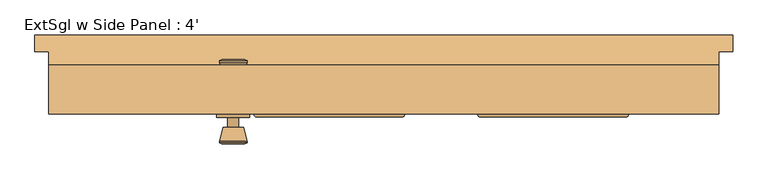
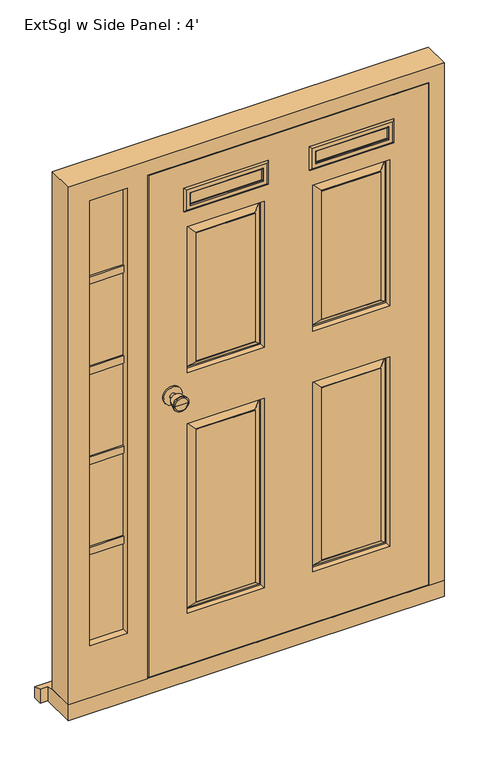
"""IFC4 building model written with IfcOpenShell, lengths in millimetres: door geometry, ExtSgl w Side Panel : 4'."""

from ifc_helpers import new_model, si_unit, point, frame, frame_2d, origin, place, context, project, spatial, polyline, circle_curve, ellipse_curve, trimmed, segment, composite_curve, outline, extrude, faceted_brep, source, transform, mapped, element, save
from ifc_brep_helpers import plane_surface, cylinder_surface, revolved_surface, advanced_brep


def extsgl_w_side_panel_4_38b62cc9(model_context):
    return source(origin(), model_context, "Body", "SolidModel", [
        advanced_brep(
        [(-493.3, -5.7, 1000.0), (-483.3, -5.7, 1000.0), (-503.3, -5.7, 1000.0), (-472.8241324, -54.7, 1000.0), (-493.3, -54.7, 1000.0), (-513.7758676, -54.7, 1000.0), (-468.3, -52.8721319, 1000.0), (-518.3, -52.8721319, 1000.0), (-468.3, -49.4084537, 1000.0), (-518.3, -49.4084537, 1000.0), (-474.663764, -24.7, 1000.0), (-511.936236, -24.7, 1000.0), (-483.3, -24.7, 1000.0), (-503.3, -24.7, 1000.0)],
        [
            (0, 1),
            (1, 2, circle_curve(frame((-493.3, -5.7, 1000.0), z_axis=(0.0, 1.0, 0.0), x_axis=(-1.0, 0.0, 0.0)), 10.0)),
            (2, 0),
            (2, 1, circle_curve(frame((-493.3, -5.7, 1000.0), z_axis=(0.0, 1.0, 0.0), x_axis=(-1.0, 0.0, 0.0)), 10.0)),
            (3, 4),
            (4, 5),
            (5, 3, circle_curve(frame((-493.3, -54.7, 1000.0), z_axis=(0.0, -1.0, 0.0), x_axis=(-1.0, 0.0, 0.0)), 20.4758676)),
            (3, 5, circle_curve(frame((-493.3, -54.7, 1000.0), z_axis=(0.0, -1.0, 0.0), x_axis=(-1.0, 0.0, 0.0)), 20.4758676)),
            (6, 3),
            (5, 7),
            (7, 6, circle_curve(frame((-493.3, -52.8721319, 1000.0), z_axis=(0.0, -1.0, 0.0), x_axis=(-1.0, 0.0, 0.0)), 25.0)),
            (6, 7, circle_curve(frame((-493.3, -52.8721319, 1000.0), z_axis=(0.0, -1.0, 0.0), x_axis=(-1.0, 0.0, 0.0)), 25.0)),
            (8, 6),
            (7, 9),
            (9, 8, circle_curve(frame((-493.3, -49.4084537, 1000.0), z_axis=(0.0, -1.0, 0.0), x_axis=(-1.0, 0.0, 0.0)), 25.0)),
            (8, 9, circle_curve(frame((-493.3, -49.4084537, 1000.0), z_axis=(0.0, -1.0, 0.0), x_axis=(-1.0, 0.0, 0.0)), 25.0)),
            (10, 8),
            (9, 11),
            (11, 10, circle_curve(frame((-493.3, -24.7, 1000.0), z_axis=(0.0, -1.0, 0.0), x_axis=(-1.0, 0.0, 0.0)), 18.636236)),
            (10, 11, circle_curve(frame((-493.3, -24.7, 1000.0), z_axis=(0.0, -1.0, 0.0), x_axis=(-1.0, 0.0, 0.0)), 18.636236)),
            (12, 10),
            (11, 13),
            (13, 12, circle_curve(frame((-493.3, -24.7, 1000.0), z_axis=(0.0, -1.0, 0.0), x_axis=(-1.0, 0.0, 0.0)), 10.0)),
            (12, 13, circle_curve(frame((-493.3, -24.7, 1000.0), z_axis=(0.0, -1.0, 0.0), x_axis=(-1.0, 0.0, 0.0)), 10.0)),
            (1, 12),
            (13, 2),
        ],
        [
            plane_surface(frame((-493.3, -5.7, 1000.0), z_axis=(0.0, 1.0, 0.0), x_axis=(-1.0, 0.0, 0.0))),
            plane_surface(frame((-493.3, -54.7, 1000.0), z_axis=(0.0, -1.0, 0.0), x_axis=(-1.0, 0.0, 0.0))),
            revolved_surface(polyline([(-513.7758676, -54.7, 1000.0), (-518.3, -52.8721319, 1000.0)]), (-493.3, -5.7, 1000.0), (0.0, 1.0, 0.0)),
            cylinder_surface(frame((-493.3, -5.7, 1000.0), z_axis=(0.0, 1.0, 0.0), x_axis=(-1.0, 0.0, 0.0)), 25.0),
            revolved_surface(polyline([(-518.3, -49.4084537, 1000.0), (-511.936236, -24.7, 1000.0)]), (-493.3, -5.7, 1000.0), (0.0, 1.0, 0.0)),
            plane_surface(frame((-493.3, -24.7, 1000.0), z_axis=(0.0, 1.0, 0.0), x_axis=(-1.0, 0.0, 0.0))),
            cylinder_surface(frame((-493.3, -5.7, 1000.0), z_axis=(0.0, 1.0, 0.0), x_axis=(-1.0, 0.0, 0.0)), 10.0),
        ],
        [
            (0, [[1, 2, 3]]),
            (0, [[-3, 4, -1]]),
            (1, [[5, 6, 7]]),
            (1, [[-6, -5, 8]]),
            (2, [[9, -7, 10, 11]]),
            (2, [[-10, -8, -9, 12]]),
            (3, [[13, -11, 14, 15]]),
            (3, [[-14, -12, -13, 16]]),
            (4, [[17, -15, 18, 19]]),
            (4, [[-18, -16, -17, 20]]),
            (5, [[21, -19, 22, 23]]),
            (5, [[-22, -20, -21, 24]]),
            (6, [[25, -23, 26, -2]]),
            (6, [[-26, -24, -25, -4]]),
        ],
    ),
        extrude(outline(composite_curve([segment(trimmed(circle_curve(frame_2d((1000.0, -493.3)), 30.0), [point((1000.0, -523.3))], [point((1000.0, -463.3))], False, "CARTESIAN"), True, "CONTINUOUS"), segment(trimmed(circle_curve(frame_2d((1000.0, -493.3)), 30.0), [point((1000.0, -463.3))], [point((1000.0, -523.3))], False, "CARTESIAN"), True, "CONTINUOUS")], self_intersect=False)), frame((0.0, -5.7, 0.0), z_axis=(0.0, 1.0, 0.0), x_axis=(0.0, 0.0, 1.0)), (0.0, 0.0, 1.0), 6.0),
        advanced_brep(
        [(-493.3, 50.3, 1000.0), (-503.3, 50.3, 1000.0), (-483.3, 50.3, 1000.0), (-472.8241324, 99.3, 1000.0), (-513.7758676, 99.3, 1000.0), (-493.3, 99.3, 1000.0), (-468.3, 97.4721319, 1000.0), (-518.3, 97.4721319, 1000.0), (-468.3, 94.0084537, 1000.0), (-518.3, 94.0084537, 1000.0), (-474.663764, 69.3, 1000.0), (-511.936236, 69.3, 1000.0), (-483.3, 69.3, 1000.0), (-503.3, 69.3, 1000.0)],
        [
            (0, 1),
            (1, 2, circle_curve(frame((-493.3, 50.3, 1000.0), z_axis=(0.0, -1.0, 0.0), x_axis=(-1.0, 0.0, 0.0)), 10.0)),
            (2, 0),
            (2, 1, circle_curve(frame((-493.3, 50.3, 1000.0), z_axis=(0.0, -1.0, 0.0), x_axis=(-1.0, 0.0, 0.0)), 10.0)),
            (3, 4, circle_curve(frame((-493.3, 99.3, 1000.0), z_axis=(0.0, 1.0, 0.0), x_axis=(-1.0, 0.0, 0.0)), 20.4758676)),
            (4, 5),
            (5, 3),
            (4, 3, circle_curve(frame((-493.3, 99.3, 1000.0), z_axis=(0.0, 1.0, 0.0), x_axis=(-1.0, 0.0, 0.0)), 20.4758676)),
            (6, 7, circle_curve(frame((-493.3, 97.4721319, 1000.0), z_axis=(0.0, 1.0, 0.0), x_axis=(-1.0, 0.0, 0.0)), 25.0)),
            (7, 4),
            (3, 6),
            (7, 6, circle_curve(frame((-493.3, 97.4721319, 1000.0), z_axis=(0.0, 1.0, 0.0), x_axis=(-1.0, 0.0, 0.0)), 25.0)),
            (8, 9, circle_curve(frame((-493.3, 94.0084537, 1000.0), z_axis=(0.0, 1.0, 0.0), x_axis=(-1.0, 0.0, 0.0)), 25.0)),
            (9, 7),
            (6, 8),
            (9, 8, circle_curve(frame((-493.3, 94.0084537, 1000.0), z_axis=(0.0, 1.0, 0.0), x_axis=(-1.0, 0.0, 0.0)), 25.0)),
            (10, 11, circle_curve(frame((-493.3, 69.3, 1000.0), z_axis=(0.0, 1.0, 0.0), x_axis=(-1.0, 0.0, 0.0)), 18.636236)),
            (11, 9),
            (8, 10),
            (11, 10, circle_curve(frame((-493.3, 69.3, 1000.0), z_axis=(0.0, 1.0, 0.0), x_axis=(-1.0, 0.0, 0.0)), 18.636236)),
            (12, 13, circle_curve(frame((-493.3, 69.3, 1000.0), z_axis=(0.0, 1.0, 0.0), x_axis=(-1.0, 0.0, 0.0)), 10.0)),
            (13, 11),
            (10, 12),
            (13, 12, circle_curve(frame((-493.3, 69.3, 1000.0), z_axis=(0.0, 1.0, 0.0), x_axis=(-1.0, 0.0, 0.0)), 10.0)),
            (1, 13),
            (12, 2),
        ],
        [
            plane_surface(frame((-493.3, 50.3, 1000.0), z_axis=(0.0, -1.0, 0.0), x_axis=(-1.0, 0.0, 0.0))),
            plane_surface(frame((-493.3, 99.3, 1000.0), z_axis=(0.0, 1.0, 0.0), x_axis=(-1.0, 0.0, 0.0))),
            revolved_surface(polyline([(-513.7758676, 99.3, 1000.0), (-518.3, 97.4721319, 1000.0)]), (-493.3, 50.3, 1000.0), (0.0, -1.0, 0.0)),
            cylinder_surface(frame((-493.3, 50.3, 1000.0), z_axis=(0.0, -1.0, 0.0), x_axis=(-1.0, 0.0, 0.0)), 25.0),
            revolved_surface(polyline([(-518.3, 94.0084537, 1000.0), (-511.936236, 69.3, 1000.0)]), (-493.3, 50.3, 1000.0), (0.0, -1.0, 0.0)),
            plane_surface(frame((-493.3, 69.3, 1000.0), z_axis=(0.0, -1.0, 0.0), x_axis=(-1.0, 0.0, 0.0))),
            cylinder_surface(frame((-493.3, 50.3, 1000.0), z_axis=(0.0, -1.0, 0.0), x_axis=(-1.0, 0.0, 0.0)), 10.0),
        ],
        [
            (0, [[1, 2, 3]]),
            (0, [[-3, 4, -1]]),
            (1, [[5, 6, 7]]),
            (1, [[8, -7, -6]]),
            (2, [[9, 10, -5, 11]]),
            (2, [[12, -11, -8, -10]]),
            (3, [[13, 14, -9, 15]]),
            (3, [[16, -15, -12, -14]]),
            (4, [[17, 18, -13, 19]]),
            (4, [[20, -19, -16, -18]]),
            (5, [[21, 22, -17, 23]]),
            (5, [[24, -23, -20, -22]]),
            (6, [[-2, 25, -21, 26]]),
            (6, [[-4, -26, -24, -25]]),
        ],
    ),
        extrude(outline(composite_curve([segment(trimmed(circle_curve(frame_2d((1000.0, -493.3)), 30.0), [point((1000.0, -523.3))], [point((1000.0, -463.3))], False, "CARTESIAN"), True, "CONTINUOUS"), segment(trimmed(circle_curve(frame_2d((1000.0, -493.3)), 30.0), [point((1000.0, -463.3))], [point((1000.0, -523.3))], False, "CARTESIAN"), True, "CONTINUOUS")], self_intersect=False)), frame((0.0, 44.3, 0.0), z_axis=(0.0, 1.0, 0.0), x_axis=(0.0, 0.0, 1.0)), (0.0, 0.0, 1.0), 6.0),
        faceted_brep([(319.7, 89.3, 54.5), (390.2, 89.3, 54.5), (390.2, 0.3, 54.5), (341.7, 0.3, 54.5), (341.7, 47.3, 54.5), (319.7, 47.3, 54.5), (319.7, 89.3, 1758.3), (-551.3, 89.3, 1758.3), (-551.3, 89.3, 54.5), (-829.0, 89.3, 54.5), (-829.0, 89.3, 1828.8), (390.2, 89.3, 1828.8), (-637.3, 89.3, 1758.3), (-758.5, 89.3, 1758.3), (-758.5, 89.3, 233.5), (-637.3, 89.3, 233.5), (390.2, 0.3, 1828.8), (-829.0, 0.3, 1828.8), (-829.0, 0.3, 54.5), (-573.3, 0.3, 54.5), (-573.3, 0.3, 1780.3), (341.7, 0.3, 1780.3), (-637.3, 0.3, 233.5), (-758.5, 0.3, 233.5), (-758.5, 0.3, 1758.3), (-637.3, 0.3, 1758.3), (341.7, 47.3, 1780.3), (-573.3, 47.3, 1780.3), (-573.3, 47.3, 54.5), (-551.3, 47.3, 54.5), (-551.3, 47.3, 1758.3), (319.7, 47.3, 1758.3), (-615.3, 47.3, 1780.3), (-780.5, 47.3, 1780.3), (-780.5, 47.3, 218.5), (-615.3, 47.3, 218.5), (-758.5, 47.3, 1758.3), (-637.3, 47.3, 1758.3), (-637.3, 47.3, 233.5), (-758.5, 47.3, 233.5), (-637.3, 23.3, 233.5), (-758.5, 23.3, 233.5), (-758.5, 23.3, 1758.3), (-637.3, 23.3, 1758.3), (-780.5, 23.3, 1780.3), (-780.5, 23.3, 218.5), (-615.3, 23.3, 218.5), (-615.3, 23.3, 1780.3)], [[[0, 1, 2, 3, 4, 5]], [[1, 0, 6, 7, 8, 9, 10, 11], [12, 13, 14, 15]], [[2, 1, 11, 16]], [[3, 2, 16, 17, 18, 19, 20, 21], [22, 23, 24, 25]], [[4, 3, 21, 26]], [[5, 4, 26, 27, 28, 29, 30, 31]], [[32, 33, 34, 35], [36, 37, 38, 39]], [[0, 5, 31, 6]], [[29, 8, 7, 30]], [[18, 9, 8, 29, 28, 19]], [[10, 9, 18, 17]], [[13, 36, 39, 14]], [[39, 38, 15, 14]], [[37, 12, 15, 38]], [[23, 22, 40, 41]], [[24, 23, 41, 42]], [[22, 25, 43, 40]], [[19, 28, 27, 20]], [[44, 45, 34, 33]], [[45, 46, 35, 34]], [[46, 47, 32, 35]], [[46, 45, 44, 47], [41, 40, 43, 42]], [[11, 10, 17, 16]], [[26, 21, 20, 27]], [[33, 32, 47, 44]], [[6, 31, 30, 7]], [[36, 13, 12, 37]], [[25, 24, 42, 43]]]),
        faceted_brep([(338.7, 0.3, 58.5), (338.7, 0.3, 1777.3), (-568.3, 0.3, 1777.3), (-568.3, 0.3, 58.5), (-36.3, 0.3, 1683.5), (213.7, 0.3, 1683.5), (213.7, 0.3, 1627.3), (-36.3, 0.3, 1627.3), (-443.3, 0.3, 1683.5), (-193.3, 0.3, 1683.5), (-193.3, 0.3, 1627.3), (-443.3, 0.3, 1627.3), (-193.3, 0.3, 883.5), (-193.3, 0.3, 233.5), (-443.3, 0.3, 233.5), (-443.3, 0.3, 883.5), (213.7, 0.3, 883.5), (213.7, 0.3, 233.5), (-36.3, 0.3, 233.5), (-36.3, 0.3, 883.5), (-193.3, 0.3, 1558.5), (-193.3, 0.3, 1058.5), (-443.3, 0.3, 1058.5), (-443.3, 0.3, 1558.5), (213.7, 0.3, 1558.5), (213.7, 0.3, 1058.5), (-36.3, 0.3, 1058.5), (-36.3, 0.3, 1558.5), (-223.3, 0.3, 263.5), (-223.3, 0.3, 853.5), (-413.3, 0.3, 853.5), (-413.3, 0.3, 263.5), (183.7, 0.3, 263.5), (183.7, 0.3, 853.5), (-6.3, 0.3, 853.5), (-6.3, 0.3, 263.5), (-223.3, 0.3, 1088.5), (-223.3, 0.3, 1528.5), (-413.3, 0.3, 1528.5), (-413.3, 0.3, 1088.5), (183.7, 0.3, 1088.5), (183.7, 0.3, 1528.5), (-6.3, 0.3, 1528.5), (-6.3, 0.3, 1088.5), (338.7, 44.3, 58.5), (-568.3, 44.3, 58.5), (-568.3, 44.3, 1777.3), (338.7, 44.3, 1777.3), (-36.3, 44.3, 1683.5), (-36.3, 44.3, 1627.3), (213.7, 44.3, 1627.3), (213.7, 44.3, 1683.5), (-443.3, 44.3, 1683.5), (-443.3, 44.3, 1627.3), (-193.3, 44.3, 1627.3), (-193.3, 44.3, 1683.5), (-36.3, 44.3, 883.5), (-36.3, 44.3, 233.5), (213.7, 44.3, 233.5), (213.7, 44.3, 883.5), (-443.3, 44.3, 883.5), (-443.3, 44.3, 233.5), (-193.3, 44.3, 233.5), (-193.3, 44.3, 883.5), (-36.3, 44.3, 1558.5), (-36.3, 44.3, 1058.5), (213.7, 44.3, 1058.5), (213.7, 44.3, 1558.5), (-443.3, 44.3, 1558.5), (-443.3, 44.3, 1058.5), (-193.3, 44.3, 1058.5), (-193.3, 44.3, 1558.5), (-6.3, 44.3, 263.5), (-6.3, 44.3, 853.5), (183.7, 44.3, 853.5), (183.7, 44.3, 263.5), (-413.3, 44.3, 263.5), (-413.3, 44.3, 853.5), (-223.3, 44.3, 853.5), (-223.3, 44.3, 263.5), (-6.3, 44.3, 1088.5), (-6.3, 44.3, 1528.5), (183.7, 44.3, 1528.5), (183.7, 44.3, 1088.5), (-413.3, 44.3, 1088.5), (-413.3, 44.3, 1528.5), (-223.3, 44.3, 1528.5), (-223.3, 44.3, 1088.5), (-33.3, 29.3, 880.5), (-33.3, 29.3, 236.5), (-8.3, 43.3, 855.5), (-8.3, 43.3, 261.5), (-28.3, 29.3, 241.5), (-28.3, 29.3, 875.5), (-6.3, 43.3, 263.5), (-6.3, 43.3, 853.5), (210.7, 29.3, 236.5), (185.7, 43.3, 261.5), (205.7, 29.3, 241.5), (183.7, 43.3, 263.5), (210.7, 29.3, 880.5), (185.7, 43.3, 855.5), (205.7, 29.3, 875.5), (183.7, 43.3, 853.5), (-440.3, 29.3, 880.5), (-440.3, 29.3, 236.5), (-415.3, 43.3, 855.5), (-415.3, 43.3, 261.5), (-435.3, 29.3, 241.5), (-435.3, 29.3, 875.5), (-413.3, 43.3, 263.5), (-413.3, 43.3, 853.5), (-196.3, 29.3, 236.5), (-221.3, 43.3, 261.5), (-201.3, 29.3, 241.5), (-223.3, 43.3, 263.5), (-196.3, 29.3, 880.5), (-221.3, 43.3, 855.5), (-201.3, 29.3, 875.5), (-223.3, 43.3, 853.5), (-223.3, 1.3, 263.5), (-223.3, 1.3, 853.5), (-201.3, 15.3, 241.5), (-201.3, 15.3, 875.5), (-221.3, 1.3, 855.5), (-221.3, 1.3, 261.5), (-196.3, 15.3, 880.5), (-196.3, 15.3, 236.5), (-413.3, 1.3, 853.5), (-435.3, 15.3, 875.5), (-415.3, 1.3, 855.5), (-440.3, 15.3, 880.5), (-413.3, 1.3, 263.5), (-435.3, 15.3, 241.5), (-415.3, 1.3, 261.5), (-440.3, 15.3, 236.5), (210.7, 15.3, 880.5), (210.7, 15.3, 236.5), (185.7, 1.3, 855.5), (185.7, 1.3, 261.5), (205.7, 15.3, 241.5), (205.7, 15.3, 875.5), (183.7, 1.3, 263.5), (183.7, 1.3, 853.5), (-33.3, 15.3, 236.5), (-8.3, 1.3, 261.5), (-28.3, 15.3, 241.5), (-6.3, 1.3, 263.5), (-33.3, 15.3, 880.5), (-8.3, 1.3, 855.5), (-28.3, 15.3, 875.5), (-6.3, 1.3, 853.5), (-6.3, 43.3, 1088.5), (-6.3, 43.3, 1528.5), (-28.3, 29.3, 1066.5), (-28.3, 29.3, 1550.5), (-8.3, 43.3, 1530.5), (-8.3, 43.3, 1086.5), (-33.3, 29.3, 1555.5), (-33.3, 29.3, 1061.5), (183.7, 43.3, 1528.5), (205.7, 29.3, 1550.5), (185.7, 43.3, 1530.5), (210.7, 29.3, 1555.5), (183.7, 43.3, 1088.5), (205.7, 29.3, 1066.5), (185.7, 43.3, 1086.5), (210.7, 29.3, 1061.5), (-413.3, 43.3, 1088.5), (-413.3, 43.3, 1528.5), (-435.3, 29.3, 1066.5), (-435.3, 29.3, 1550.5), (-415.3, 43.3, 1530.5), (-415.3, 43.3, 1086.5), (-440.3, 29.3, 1555.5), (-440.3, 29.3, 1061.5), (-223.3, 43.3, 1528.5), (-201.3, 29.3, 1550.5), (-221.3, 43.3, 1530.5), (-196.3, 29.3, 1555.5), (-223.3, 43.3, 1088.5), (-201.3, 29.3, 1066.5), (-221.3, 43.3, 1086.5), (-196.3, 29.3, 1061.5), (-223.3, 1.3, 1088.5), (-223.3, 1.3, 1528.5), (-201.3, 15.3, 1066.5), (-201.3, 15.3, 1550.5), (-221.3, 1.3, 1530.5), (-221.3, 1.3, 1086.5), (-196.3, 15.3, 1555.5), (-196.3, 15.3, 1061.5), (-413.3, 1.3, 1528.5), (-435.3, 15.3, 1550.5), (-415.3, 1.3, 1530.5), (-440.3, 15.3, 1555.5), (-413.3, 1.3, 1088.5), (-435.3, 15.3, 1066.5), (-415.3, 1.3, 1086.5), (-440.3, 15.3, 1061.5), (210.7, 15.3, 1555.5), (210.7, 15.3, 1061.5), (185.7, 1.3, 1530.5), (185.7, 1.3, 1086.5), (205.7, 15.3, 1066.5), (205.7, 15.3, 1550.5), (183.7, 1.3, 1088.5), (183.7, 1.3, 1528.5), (-33.3, 15.3, 1061.5), (-8.3, 1.3, 1086.5), (-28.3, 15.3, 1066.5), (-6.3, 1.3, 1088.5), (-33.3, 15.3, 1555.5), (-8.3, 1.3, 1530.5), (-28.3, 15.3, 1550.5), (-6.3, 1.3, 1528.5)], [[[0, 1, 2, 3], [4, 5, 6, 7], [8, 9, 10, 11], [12, 13, 14, 15], [16, 17, 18, 19], [20, 21, 22, 23], [24, 25, 26, 27]], [[28, 29, 30, 31]], [[32, 33, 34, 35]], [[36, 37, 38, 39]], [[40, 41, 42, 43]], [[44, 45, 46, 47], [48, 49, 50, 51], [52, 53, 54, 55], [56, 57, 58, 59], [60, 61, 62, 63], [64, 65, 66, 67], [68, 69, 70, 71]], [[72, 73, 74, 75]], [[76, 77, 78, 79]], [[80, 81, 82, 83]], [[84, 85, 86, 87]], [[1, 0, 44, 47]], [[2, 1, 47, 46]], [[3, 2, 46, 45]], [[0, 3, 45, 44]], [[4, 7, 49, 48]], [[7, 6, 50, 49]], [[6, 5, 51, 50]], [[5, 4, 48, 51]], [[8, 11, 53, 52]], [[11, 10, 54, 53]], [[10, 9, 55, 54]], [[9, 8, 52, 55]], [[88, 89, 57, 56]], [[90, 91, 92, 93]], [[72, 94, 95, 73]], [[57, 89, 96, 58]], [[92, 91, 97, 98]], [[94, 72, 75, 99]], [[58, 96, 100, 59]], [[98, 97, 101, 102]], [[99, 75, 74, 103]], [[88, 56, 59, 100]], [[89, 88, 100, 96], [93, 92, 98, 102]], [[90, 93, 102, 101]], [[91, 90, 101, 97], [95, 94, 99, 103]], [[73, 95, 103, 74]], [[104, 105, 61, 60]], [[106, 107, 108, 109]], [[76, 110, 111, 77]], [[61, 105, 112, 62]], [[108, 107, 113, 114]], [[110, 76, 79, 115]], [[62, 112, 116, 63]], [[114, 113, 117, 118]], [[115, 79, 78, 119]], [[104, 60, 63, 116]], [[105, 104, 116, 112], [109, 108, 114, 118]], [[106, 109, 118, 117]], [[107, 106, 117, 113], [111, 110, 115, 119]], [[77, 111, 119, 78]], [[120, 121, 29, 28]], [[122, 123, 124, 125]], [[12, 126, 127, 13]], [[29, 121, 128, 30]], [[124, 123, 129, 130]], [[126, 12, 15, 131]], [[30, 128, 132, 31]], [[130, 129, 133, 134]], [[131, 15, 14, 135]], [[120, 28, 31, 132]], [[125, 124, 130, 134], [121, 120, 132, 128]], [[122, 125, 134, 133]], [[127, 126, 131, 135], [123, 122, 133, 129]], [[13, 127, 135, 14]], [[136, 137, 17, 16]], [[138, 139, 140, 141]], [[32, 142, 143, 33]], [[17, 137, 144, 18]], [[140, 139, 145, 146]], [[142, 32, 35, 147]], [[18, 144, 148, 19]], [[146, 145, 149, 150]], [[147, 35, 34, 151]], [[136, 16, 19, 148]], [[137, 136, 148, 144], [141, 140, 146, 150]], [[138, 141, 150, 149]], [[139, 138, 149, 145], [143, 142, 147, 151]], [[33, 143, 151, 34]], [[152, 153, 81, 80]], [[154, 155, 156, 157]], [[64, 158, 159, 65]], [[81, 153, 160, 82]], [[156, 155, 161, 162]], [[158, 64, 67, 163]], [[82, 160, 164, 83]], [[162, 161, 165, 166]], [[163, 67, 66, 167]], [[152, 80, 83, 164]], [[157, 156, 162, 166], [153, 152, 164, 160]], [[154, 157, 166, 165]], [[159, 158, 163, 167], [155, 154, 165, 161]], [[65, 159, 167, 66]], [[168, 169, 85, 84]], [[170, 171, 172, 173]], [[68, 174, 175, 69]], [[85, 169, 176, 86]], [[172, 171, 177, 178]], [[174, 68, 71, 179]], [[86, 176, 180, 87]], [[178, 177, 181, 182]], [[179, 71, 70, 183]], [[168, 84, 87, 180]], [[173, 172, 178, 182], [169, 168, 180, 176]], [[170, 173, 182, 181]], [[175, 174, 179, 183], [171, 170, 181, 177]], [[69, 175, 183, 70]], [[184, 185, 37, 36]], [[186, 187, 188, 189]], [[20, 190, 191, 21]], [[37, 185, 192, 38]], [[188, 187, 193, 194]], [[190, 20, 23, 195]], [[38, 192, 196, 39]], [[194, 193, 197, 198]], [[195, 23, 22, 199]], [[184, 36, 39, 196]], [[189, 188, 194, 198], [185, 184, 196, 192]], [[186, 189, 198, 197]], [[191, 190, 195, 199], [187, 186, 197, 193]], [[21, 191, 199, 22]], [[200, 201, 25, 24]], [[202, 203, 204, 205]], [[40, 206, 207, 41]], [[25, 201, 208, 26]], [[204, 203, 209, 210]], [[206, 40, 43, 211]], [[26, 208, 212, 27]], [[210, 209, 213, 214]], [[211, 43, 42, 215]], [[200, 24, 27, 212]], [[201, 200, 212, 208], [205, 204, 210, 214]], [[202, 205, 214, 213]], [[203, 202, 213, 209], [207, 206, 211, 215]], [[41, 207, 215, 42]]]),
        faceted_brep([(415.2, 144.3, 0.0), (415.2, 144.3, 38.5947221), (415.2, 114.3, 47.2703282), (415.2, 114.3, 0.0), (-854.0, 144.3, 38.5947221), (-854.0, 144.3, 0.0), (-854.0, 114.3, 0.0), (-854.0, 114.3, 47.2703282), (390.2, 114.3, 0.0), (390.2, 0.3, 0.0), (-829.0, 0.3, 0.0), (-829.0, 114.3, 0.0), (-829.0, 114.3, 47.2703282), (-829.0, 89.3, 54.5), (390.2, 89.3, 54.5), (390.2, 114.3, 47.2703282), (-829.0, 0.3, 54.5), (390.2, 0.3, 54.5)], [[[0, 1, 2, 3]], [[4, 5, 6, 7]], [[5, 0, 3, 8, 9, 10, 11, 6]], [[1, 0, 5, 4]], [[1, 4, 7, 12, 13, 14, 15, 2]], [[13, 16, 17, 14]], [[16, 10, 9, 17]], [[12, 11, 10, 16, 13]], [[11, 12, 7, 6]], [[8, 15, 14, 17, 9]], [[15, 8, 3, 2]]]),
        extrude(outline(polyline([(213.7, 10.3), (-36.3, 10.3), (-36.3, 34.3), (213.7, 34.3), (213.7, 10.3)])), frame((0.0, 0.0, 1627.3), z_axis=(0.0, 0.0, 1.0), x_axis=(1.0, 0.0, 0.0)), (0.0, 0.0, 1.0), 56.2),
        extrude(outline(polyline([(-193.3, 10.3), (-443.3, 10.3), (-443.3, 34.3), (-193.3, 34.3), (-193.3, 10.3)])), frame((0.0, 0.0, 1627.3), z_axis=(0.0, 0.0, 1.0), x_axis=(1.0, 0.0, 0.0)), (0.0, 0.0, 1.0), 56.2),
        advanced_brep(
        [(-28.3, 48.3, 1675.5), (-28.3, 44.3, 1675.5), (-28.3, 44.3, 1635.3), (-28.3, 48.3, 1635.3), (-30.3, 50.3, 1677.5), (-30.3, 50.3, 1633.3), (-48.3, 45.3, 1695.5), (-43.3, 50.3, 1690.5), (-43.3, 50.3, 1620.3), (-48.3, 45.3, 1615.3), (-48.3, 34.3, 1695.5), (-48.3, 34.3, 1615.3), (-36.3, 44.3, 1683.5), (-36.3, 34.3, 1683.5), (-36.3, 34.3, 1627.3), (-36.3, 44.3, 1627.3), (205.7, 44.3, 1635.3), (205.7, 48.3, 1635.3), (207.7, 50.3, 1633.3), (220.7, 50.3, 1620.3), (225.7, 45.3, 1615.3), (225.7, 34.3, 1615.3), (213.7, 34.3, 1627.3), (213.7, 44.3, 1627.3), (205.7, 44.3, 1675.5), (205.7, 48.3, 1675.5), (207.7, 50.3, 1677.5), (220.7, 50.3, 1690.5), (225.7, 45.3, 1695.5), (225.7, 34.3, 1695.5), (213.7, 34.3, 1683.5), (213.7, 44.3, 1683.5)],
        [
            (0, 1),
            (1, 2),
            (2, 3),
            (3, 0),
            (4, 0, ellipse_curve(frame((-30.3, 48.3, 1677.5), z_axis=(-0.7071067811865475, 0.0, -0.7071067811865475), x_axis=(-0.7071067811865474, 0.0, 0.7071067811865476)), 2.8284271, 2.0)),
            (3, 5, ellipse_curve(frame((-30.3, 48.3, 1633.3), z_axis=(-0.7071067811865475, 0.0, 0.7071067811865475), x_axis=(0.7071067811865474, 0.0, 0.7071067811865476)), 2.8284271, 2.0)),
            (5, 4),
            (6, 7, ellipse_curve(frame((-43.3, 45.3, 1690.5), z_axis=(-0.7071067811865475, 0.0, -0.7071067811865475), x_axis=(-0.7071067811865474, 0.0, 0.7071067811865476)), 7.0710678, 5.0)),
            (7, 8),
            (8, 9, ellipse_curve(frame((-43.3, 45.3, 1620.3), z_axis=(-0.7071067811865475, 0.0, 0.7071067811865475), x_axis=(0.7071067811865474, 0.0, 0.7071067811865476)), 7.0710678, 5.0)),
            (9, 6),
            (10, 6),
            (9, 11),
            (11, 10),
            (12, 13),
            (13, 14),
            (14, 15),
            (15, 12),
            (2, 16),
            (16, 17),
            (17, 3),
            (17, 18, ellipse_curve(frame((207.7, 48.3, 1633.3), z_axis=(-0.7071067811865475, 0.0, -0.7071067811865475), x_axis=(-0.7071067811865476, 0.0, 0.7071067811865474)), 2.8284271, 2.0)),
            (18, 5),
            (8, 19),
            (19, 20, ellipse_curve(frame((220.7, 45.3, 1620.3), z_axis=(-0.7071067811865475, 0.0, -0.7071067811865475), x_axis=(-0.7071067811865476, 0.0, 0.7071067811865474)), 7.0710678, 5.0)),
            (20, 9),
            (20, 21),
            (21, 11),
            (14, 22),
            (22, 23),
            (23, 15),
            (16, 24),
            (24, 25),
            (25, 17),
            (25, 26, ellipse_curve(frame((207.7, 48.3, 1677.5), z_axis=(0.7071067811865475, 0.0, -0.7071067811865475), x_axis=(-0.7071067811865474, 0.0, -0.7071067811865476)), 2.8284271, 2.0)),
            (26, 18),
            (19, 27),
            (27, 28, ellipse_curve(frame((220.7, 45.3, 1690.5), z_axis=(0.7071067811865475, 0.0, -0.7071067811865475), x_axis=(-0.7071067811865474, 0.0, -0.7071067811865476)), 7.0710678, 5.0)),
            (28, 20),
            (28, 29),
            (29, 21),
            (22, 30),
            (30, 31),
            (31, 23),
            (24, 1),
            (0, 25),
            (4, 26),
            (7, 27),
            (6, 28),
            (10, 29),
            (13, 30),
            (12, 31),
        ],
        [
            plane_surface(frame((-28.3, 44.3, 1675.5), z_axis=(1.0, 0.0, 0.0), x_axis=(0.0, 0.0, -1.0))),
            cylinder_surface(frame((-30.3, 48.3, 1683.5), z_axis=(0.0, 0.0, 1.0), x_axis=(1.0, 0.0, 0.0)), 2.0),
            cylinder_surface(frame((-43.3, 45.3, 1683.5), z_axis=(0.0, 0.0, 1.0), x_axis=(1.0, 0.0, 0.0)), 5.0),
            plane_surface(frame((-48.3, 45.3, 1695.5), z_axis=(-1.0, 0.0, 0.0), x_axis=(0.0, 0.0, -1.0))),
            plane_surface(frame((-36.3, 34.3, 1683.5), z_axis=(1.0, 0.0, 0.0), x_axis=(0.0, 0.0, -1.0))),
            plane_surface(frame((-28.3, 44.3, 1635.3), z_axis=(0.0, 0.0, 1.0), x_axis=(1.0, 0.0, 0.0))),
            cylinder_surface(frame((-36.3, 48.3, 1633.3), z_axis=(-1.0, 0.0, 0.0), x_axis=(0.0, 0.0, 1.0)), 2.0),
            cylinder_surface(frame((-36.3, 45.3, 1620.3), z_axis=(-1.0, 0.0, 0.0), x_axis=(0.0, 0.0, 1.0)), 5.0),
            plane_surface(frame((-48.3, 45.3, 1615.3), z_axis=(0.0, 0.0, -1.0), x_axis=(1.0, 0.0, 0.0))),
            plane_surface(frame((-36.3, 34.3, 1627.3), z_axis=(0.0, 0.0, 1.0), x_axis=(1.0, 0.0, 0.0))),
            plane_surface(frame((205.7, 44.3, 1635.3), z_axis=(-1.0, 0.0, 0.0), x_axis=(0.0, 0.0, 1.0))),
            cylinder_surface(frame((207.7, 48.3, 1627.3), z_axis=(0.0, 0.0, -1.0), x_axis=(-1.0, 0.0, 0.0)), 2.0),
            cylinder_surface(frame((220.7, 45.3, 1627.3), z_axis=(0.0, 0.0, -1.0), x_axis=(-1.0, 0.0, 0.0)), 5.0),
            plane_surface(frame((225.7, 45.3, 1615.3), z_axis=(1.0, 0.0, 0.0), x_axis=(0.0, 0.0, 1.0))),
            plane_surface(frame((213.7, 34.3, 1627.3), z_axis=(-1.0, 0.0, 0.0), x_axis=(0.0, 0.0, 1.0))),
            plane_surface(frame((205.7, 44.3, 1675.5), z_axis=(0.0, 0.0, -1.0), x_axis=(-1.0, 0.0, 0.0))),
            cylinder_surface(frame((213.7, 48.3, 1677.5), z_axis=(1.0, 0.0, 0.0), x_axis=(0.0, 0.0, -1.0)), 2.0),
            plane_surface(frame((207.7, 50.3, 1677.5), z_axis=(0.0, 1.0, 0.0), x_axis=(-1.0, 0.0, 0.0))),
            cylinder_surface(frame((213.7, 45.3, 1690.5), z_axis=(1.0, 0.0, 0.0), x_axis=(0.0, 0.0, -1.0)), 5.0),
            plane_surface(frame((225.7, 45.3, 1695.5), z_axis=(0.0, 0.0, 1.0), x_axis=(-1.0, 0.0, 0.0))),
            plane_surface(frame((225.7, 34.3, 1695.5), z_axis=(0.0, -1.0, 0.0), x_axis=(-1.0, 0.0, 0.0))),
            plane_surface(frame((213.7, 34.3, 1683.5), z_axis=(0.0, 0.0, -1.0), x_axis=(-1.0, 0.0, 0.0))),
            plane_surface(frame((213.7, 44.3, 1683.5), z_axis=(0.0, -1.0, 0.0), x_axis=(-1.0, 0.0, 0.0))),
        ],
        [
            (0, [[1, 2, 3, 4]]),
            (1, [[5, -4, 6, 7]]),
            (2, [[8, 9, 10, 11]]),
            (3, [[12, -11, 13, 14]]),
            (4, [[15, 16, 17, 18]]),
            (5, [[-3, 19, 20, 21]]),
            (6, [[-6, -21, 22, 23]]),
            (7, [[-10, 24, 25, 26]]),
            (8, [[-13, -26, 27, 28]]),
            (9, [[-17, 29, 30, 31]]),
            (10, [[-20, 32, 33, 34]]),
            (11, [[-22, -34, 35, 36]]),
            (12, [[-25, 37, 38, 39]]),
            (13, [[-27, -39, 40, 41]]),
            (14, [[-30, 42, 43, 44]]),
            (15, [[-33, 45, -1, 46]]),
            (16, [[-35, -46, -5, 47]]),
            (17, [[48, -37, -24, -9], [-23, -36, -47, -7]]),
            (18, [[-38, -48, -8, 49]]),
            (19, [[-40, -49, -12, 50]]),
            (20, [[-28, -41, -50, -14], [51, -42, -29, -16]]),
            (21, [[-43, -51, -15, 52]]),
            (22, [[-31, -44, -52, -18], [-45, -32, -19, -2]]),
        ],
    ),
        advanced_brep(
        [(-435.3, 48.3, 1675.5), (-435.3, 44.3, 1675.5), (-435.3, 44.3, 1635.3), (-435.3, 48.3, 1635.3), (-437.3, 50.3, 1677.5), (-437.3, 50.3, 1633.3), (-455.3, 45.3, 1695.5), (-450.3, 50.3, 1690.5), (-450.3, 50.3, 1620.3), (-455.3, 45.3, 1615.3), (-455.3, 34.3, 1695.5), (-455.3, 34.3, 1615.3), (-443.3, 44.3, 1683.5), (-443.3, 34.3, 1683.5), (-443.3, 34.3, 1627.3), (-443.3, 44.3, 1627.3), (-201.3, 44.3, 1635.3), (-201.3, 48.3, 1635.3), (-199.3, 50.3, 1633.3), (-186.3, 50.3, 1620.3), (-181.3, 45.3, 1615.3), (-181.3, 34.3, 1615.3), (-193.3, 34.3, 1627.3), (-193.3, 44.3, 1627.3), (-201.3, 44.3, 1675.5), (-201.3, 48.3, 1675.5), (-199.3, 50.3, 1677.5), (-186.3, 50.3, 1690.5), (-181.3, 45.3, 1695.5), (-181.3, 34.3, 1695.5), (-193.3, 34.3, 1683.5), (-193.3, 44.3, 1683.5)],
        [
            (0, 1),
            (1, 2),
            (2, 3),
            (3, 0),
            (4, 0, ellipse_curve(frame((-437.3, 48.3, 1677.5), z_axis=(-0.7071067811865475, 0.0, -0.7071067811865475), x_axis=(-0.7071067811865474, 0.0, 0.7071067811865476)), 2.8284271, 2.0)),
            (3, 5, ellipse_curve(frame((-437.3, 48.3, 1633.3), z_axis=(-0.7071067811865475, 0.0, 0.7071067811865475), x_axis=(0.7071067811865474, 0.0, 0.7071067811865476)), 2.8284271, 2.0)),
            (5, 4),
            (6, 7, ellipse_curve(frame((-450.3, 45.3, 1690.5), z_axis=(-0.7071067811865475, 0.0, -0.7071067811865475), x_axis=(-0.7071067811865474, 0.0, 0.7071067811865476)), 7.0710678, 5.0)),
            (7, 8),
            (8, 9, ellipse_curve(frame((-450.3, 45.3, 1620.3), z_axis=(-0.7071067811865475, 0.0, 0.7071067811865475), x_axis=(0.7071067811865474, 0.0, 0.7071067811865476)), 7.0710678, 5.0)),
            (9, 6),
            (10, 6),
            (9, 11),
            (11, 10),
            (12, 13),
            (13, 14),
            (14, 15),
            (15, 12),
            (2, 16),
            (16, 17),
            (17, 3),
            (17, 18, ellipse_curve(frame((-199.3, 48.3, 1633.3), z_axis=(-0.7071067811865475, 0.0, -0.7071067811865475), x_axis=(-0.7071067811865476, 0.0, 0.7071067811865474)), 2.8284271, 2.0)),
            (18, 5),
            (8, 19),
            (19, 20, ellipse_curve(frame((-186.3, 45.3, 1620.3), z_axis=(-0.7071067811865475, 0.0, -0.7071067811865475), x_axis=(-0.7071067811865476, 0.0, 0.7071067811865474)), 7.0710678, 5.0)),
            (20, 9),
            (20, 21),
            (21, 11),
            (14, 22),
            (22, 23),
            (23, 15),
            (16, 24),
            (24, 25),
            (25, 17),
            (25, 26, ellipse_curve(frame((-199.3, 48.3, 1677.5), z_axis=(0.7071067811865475, 0.0, -0.7071067811865475), x_axis=(-0.7071067811865474, 0.0, -0.7071067811865476)), 2.8284271, 2.0)),
            (26, 18),
            (19, 27),
            (27, 28, ellipse_curve(frame((-186.3, 45.3, 1690.5), z_axis=(0.7071067811865475, 0.0, -0.7071067811865475), x_axis=(-0.7071067811865474, 0.0, -0.7071067811865476)), 7.0710678, 5.0)),
            (28, 20),
            (28, 29),
            (29, 21),
            (22, 30),
            (30, 31),
            (31, 23),
            (24, 1),
            (0, 25),
            (4, 26),
            (7, 27),
            (6, 28),
            (10, 29),
            (13, 30),
            (12, 31),
        ],
        [
            plane_surface(frame((-435.3, 44.3, 1675.5), z_axis=(1.0, 0.0, 0.0), x_axis=(0.0, 0.0, -1.0))),
            cylinder_surface(frame((-437.3, 48.3, 1683.5), z_axis=(0.0, 0.0, 1.0), x_axis=(1.0, 0.0, 0.0)), 2.0),
            cylinder_surface(frame((-450.3, 45.3, 1683.5), z_axis=(0.0, 0.0, 1.0), x_axis=(1.0, 0.0, 0.0)), 5.0),
            plane_surface(frame((-455.3, 45.3, 1695.5), z_axis=(-1.0, 0.0, 0.0), x_axis=(0.0, 0.0, -1.0))),
            plane_surface(frame((-443.3, 34.3, 1683.5), z_axis=(1.0, 0.0, 0.0), x_axis=(0.0, 0.0, -1.0))),
            plane_surface(frame((-435.3, 44.3, 1635.3), z_axis=(0.0, 0.0, 1.0), x_axis=(1.0, 0.0, 0.0))),
            cylinder_surface(frame((-443.3, 48.3, 1633.3), z_axis=(-1.0, 0.0, 0.0), x_axis=(0.0, 0.0, 1.0)), 2.0),
            cylinder_surface(frame((-443.3, 45.3, 1620.3), z_axis=(-1.0, 0.0, 0.0), x_axis=(0.0, 0.0, 1.0)), 5.0),
            plane_surface(frame((-455.3, 45.3, 1615.3), z_axis=(0.0, 0.0, -1.0), x_axis=(1.0, 0.0, 0.0))),
            plane_surface(frame((-443.3, 34.3, 1627.3), z_axis=(0.0, 0.0, 1.0), x_axis=(1.0, 0.0, 0.0))),
            plane_surface(frame((-201.3, 44.3, 1635.3), z_axis=(-1.0, 0.0, 0.0), x_axis=(0.0, 0.0, 1.0))),
            cylinder_surface(frame((-199.3, 48.3, 1627.3), z_axis=(0.0, 0.0, -1.0), x_axis=(-1.0, 0.0, 0.0)), 2.0),
            cylinder_surface(frame((-186.3, 45.3, 1627.3), z_axis=(0.0, 0.0, -1.0), x_axis=(-1.0, 0.0, 0.0)), 5.0),
            plane_surface(frame((-181.3, 45.3, 1615.3), z_axis=(1.0, 0.0, 0.0), x_axis=(0.0, 0.0, 1.0))),
            plane_surface(frame((-193.3, 34.3, 1627.3), z_axis=(-1.0, 0.0, 0.0), x_axis=(0.0, 0.0, 1.0))),
            plane_surface(frame((-201.3, 44.3, 1675.5), z_axis=(0.0, 0.0, -1.0), x_axis=(-1.0, 0.0, 0.0))),
            cylinder_surface(frame((-193.3, 48.3, 1677.5), z_axis=(1.0, 0.0, 0.0), x_axis=(0.0, 0.0, -1.0)), 2.0),
            plane_surface(frame((-199.3, 50.3, 1677.5), z_axis=(0.0, 1.0, 0.0), x_axis=(-1.0, 0.0, 0.0))),
            cylinder_surface(frame((-193.3, 45.3, 1690.5), z_axis=(1.0, 0.0, 0.0), x_axis=(0.0, 0.0, -1.0)), 5.0),
            plane_surface(frame((-181.3, 45.3, 1695.5), z_axis=(0.0, 0.0, 1.0), x_axis=(-1.0, 0.0, 0.0))),
            plane_surface(frame((-181.3, 34.3, 1695.5), z_axis=(0.0, -1.0, 0.0), x_axis=(-1.0, 0.0, 0.0))),
            plane_surface(frame((-193.3, 34.3, 1683.5), z_axis=(0.0, 0.0, -1.0), x_axis=(-1.0, 0.0, 0.0))),
            plane_surface(frame((-193.3, 44.3, 1683.5), z_axis=(0.0, -1.0, 0.0), x_axis=(-1.0, 0.0, 0.0))),
        ],
        [
            (0, [[1, 2, 3, 4]]),
            (1, [[5, -4, 6, 7]]),
            (2, [[8, 9, 10, 11]]),
            (3, [[12, -11, 13, 14]]),
            (4, [[15, 16, 17, 18]]),
            (5, [[-3, 19, 20, 21]]),
            (6, [[-6, -21, 22, 23]]),
            (7, [[-10, 24, 25, 26]]),
            (8, [[-13, -26, 27, 28]]),
            (9, [[-17, 29, 30, 31]]),
            (10, [[-20, 32, 33, 34]]),
            (11, [[-22, -34, 35, 36]]),
            (12, [[-25, 37, 38, 39]]),
            (13, [[-27, -39, 40, 41]]),
            (14, [[-30, 42, 43, 44]]),
            (15, [[-33, 45, -1, 46]]),
            (16, [[-35, -46, -5, 47]]),
            (17, [[48, -37, -24, -9], [-23, -36, -47, -7]]),
            (18, [[-38, -48, -8, 49]]),
            (19, [[-40, -49, -12, 50]]),
            (20, [[-28, -41, -50, -14], [51, -42, -29, -16]]),
            (21, [[-43, -51, -15, 52]]),
            (22, [[-31, -44, -52, -18], [-45, -32, -19, -2]]),
        ],
    ),
        advanced_brep(
        [(-201.3, -3.7, 1675.5), (-201.3, 0.3, 1675.5), (-201.3, 0.3, 1635.3), (-201.3, -3.7, 1635.3), (-199.3, -5.7, 1677.5), (-199.3, -5.7, 1633.3), (-181.3, -0.7, 1695.5), (-186.3, -5.7, 1690.5), (-186.3, -5.7, 1620.3), (-181.3, -0.7, 1615.3), (-181.3, 10.3, 1695.5), (-181.3, 10.3, 1615.3), (-193.3, 0.3, 1683.5), (-193.3, 10.3, 1683.5), (-193.3, 10.3, 1627.3), (-193.3, 0.3, 1627.3), (-435.3, 0.3, 1635.3), (-435.3, -3.7, 1635.3), (-437.3, -5.7, 1633.3), (-450.3, -5.7, 1620.3), (-455.3, -0.7, 1615.3), (-455.3, 10.3, 1615.3), (-443.3, 10.3, 1627.3), (-443.3, 0.3, 1627.3), (-435.3, 0.3, 1675.5), (-435.3, -3.7, 1675.5), (-437.3, -5.7, 1677.5), (-450.3, -5.7, 1690.5), (-455.3, -0.7, 1695.5), (-455.3, 10.3, 1695.5), (-443.3, 10.3, 1683.5), (-443.3, 0.3, 1683.5)],
        [
            (0, 1),
            (1, 2),
            (2, 3),
            (3, 0),
            (4, 0, ellipse_curve(frame((-199.3, -3.7, 1677.5), z_axis=(0.7071067811865475, 0.0, -0.7071067811865475), x_axis=(0.7071067811865474, 0.0, 0.7071067811865476)), 2.8284271, 2.0)),
            (3, 5, ellipse_curve(frame((-199.3, -3.7, 1633.3), z_axis=(0.7071067811865475, 0.0, 0.7071067811865475), x_axis=(-0.7071067811865474, 0.0, 0.7071067811865476)), 2.8284271, 2.0)),
            (5, 4),
            (6, 7, ellipse_curve(frame((-186.3, -0.7, 1690.5), z_axis=(0.7071067811865475, 0.0, -0.7071067811865475), x_axis=(0.7071067811865474, 0.0, 0.7071067811865476)), 7.0710678, 5.0)),
            (7, 8),
            (8, 9, ellipse_curve(frame((-186.3, -0.7, 1620.3), z_axis=(0.7071067811865475, 0.0, 0.7071067811865475), x_axis=(-0.7071067811865474, 0.0, 0.7071067811865476)), 7.0710678, 5.0)),
            (9, 6),
            (10, 6),
            (9, 11),
            (11, 10),
            (12, 13),
            (13, 14),
            (14, 15),
            (15, 12),
            (2, 16),
            (16, 17),
            (17, 3),
            (17, 18, ellipse_curve(frame((-437.3, -3.7, 1633.3), z_axis=(0.7071067811865475, 0.0, -0.7071067811865475), x_axis=(0.7071067811865476, 0.0, 0.7071067811865474)), 2.8284271, 2.0)),
            (18, 5),
            (8, 19),
            (19, 20, ellipse_curve(frame((-450.3, -0.7, 1620.3), z_axis=(0.7071067811865475, 0.0, -0.7071067811865475), x_axis=(0.7071067811865476, 0.0, 0.7071067811865474)), 7.0710678, 5.0)),
            (20, 9),
            (20, 21),
            (21, 11),
            (14, 22),
            (22, 23),
            (23, 15),
            (16, 24),
            (24, 25),
            (25, 17),
            (25, 26, ellipse_curve(frame((-437.3, -3.7, 1677.5), z_axis=(-0.7071067811865475, 0.0, -0.7071067811865475), x_axis=(0.7071067811865474, 0.0, -0.7071067811865476)), 2.8284271, 2.0)),
            (26, 18),
            (19, 27),
            (27, 28, ellipse_curve(frame((-450.3, -0.7, 1690.5), z_axis=(-0.7071067811865475, 0.0, -0.7071067811865475), x_axis=(0.7071067811865474, 0.0, -0.7071067811865476)), 7.0710678, 5.0)),
            (28, 20),
            (28, 29),
            (29, 21),
            (22, 30),
            (30, 31),
            (31, 23),
            (24, 1),
            (0, 25),
            (4, 26),
            (7, 27),
            (6, 28),
            (10, 29),
            (13, 30),
            (12, 31),
        ],
        [
            plane_surface(frame((-201.3, 0.3, 1675.5), z_axis=(-1.0, 0.0, 0.0), x_axis=(0.0, 0.0, -1.0))),
            cylinder_surface(frame((-199.3, -3.7, 1683.5), z_axis=(0.0, 0.0, 1.0), x_axis=(-1.0, 0.0, 0.0)), 2.0),
            cylinder_surface(frame((-186.3, -0.7, 1683.5), z_axis=(0.0, 0.0, 1.0), x_axis=(-1.0, 0.0, 0.0)), 5.0),
            plane_surface(frame((-181.3, -0.7, 1695.5), z_axis=(1.0, 0.0, 0.0), x_axis=(0.0, 0.0, -1.0))),
            plane_surface(frame((-193.3, 10.3, 1683.5), z_axis=(-1.0, 0.0, 0.0), x_axis=(0.0, 0.0, -1.0))),
            plane_surface(frame((-201.3, 0.3, 1635.3), z_axis=(0.0, 0.0, 1.0), x_axis=(-1.0, 0.0, 0.0))),
            cylinder_surface(frame((-193.3, -3.7, 1633.3), z_axis=(1.0, 0.0, 0.0), x_axis=(0.0, 0.0, 1.0)), 2.0),
            cylinder_surface(frame((-193.3, -0.7, 1620.3), z_axis=(1.0, 0.0, 0.0), x_axis=(0.0, 0.0, 1.0)), 5.0),
            plane_surface(frame((-181.3, -0.7, 1615.3), z_axis=(0.0, 0.0, -1.0), x_axis=(-1.0, 0.0, 0.0))),
            plane_surface(frame((-193.3, 10.3, 1627.3), z_axis=(0.0, 0.0, 1.0), x_axis=(-1.0, 0.0, 0.0))),
            plane_surface(frame((-435.3, 0.3, 1635.3), z_axis=(1.0, 0.0, 0.0), x_axis=(0.0, 0.0, 1.0))),
            cylinder_surface(frame((-437.3, -3.7, 1627.3), z_axis=(0.0, 0.0, -1.0), x_axis=(1.0, 0.0, 0.0)), 2.0),
            cylinder_surface(frame((-450.3, -0.7, 1627.3), z_axis=(0.0, 0.0, -1.0), x_axis=(1.0, 0.0, 0.0)), 5.0),
            plane_surface(frame((-455.3, -0.7, 1615.3), z_axis=(-1.0, 0.0, 0.0), x_axis=(0.0, 0.0, 1.0))),
            plane_surface(frame((-443.3, 10.3, 1627.3), z_axis=(1.0, 0.0, 0.0), x_axis=(0.0, 0.0, 1.0))),
            plane_surface(frame((-435.3, 0.3, 1675.5), z_axis=(0.0, 0.0, -1.0), x_axis=(1.0, 0.0, 0.0))),
            cylinder_surface(frame((-443.3, -3.7, 1677.5), z_axis=(-1.0, 0.0, 0.0), x_axis=(0.0, 0.0, -1.0)), 2.0),
            plane_surface(frame((-437.3, -5.7, 1677.5), z_axis=(0.0, -1.0, 0.0), x_axis=(1.0, 0.0, 0.0))),
            cylinder_surface(frame((-443.3, -0.7, 1690.5), z_axis=(-1.0, 0.0, 0.0), x_axis=(0.0, 0.0, -1.0)), 5.0),
            plane_surface(frame((-455.3, -0.7, 1695.5), z_axis=(0.0, 0.0, 1.0), x_axis=(1.0, 0.0, 0.0))),
            plane_surface(frame((-455.3, 10.3, 1695.5), z_axis=(0.0, 1.0, 0.0), x_axis=(1.0, 0.0, 0.0))),
            plane_surface(frame((-443.3, 10.3, 1683.5), z_axis=(0.0, 0.0, -1.0), x_axis=(1.0, 0.0, 0.0))),
            plane_surface(frame((-443.3, 0.3, 1683.5), z_axis=(0.0, 1.0, 0.0), x_axis=(1.0, 0.0, 0.0))),
        ],
        [
            (0, [[1, 2, 3, 4]]),
            (1, [[5, -4, 6, 7]]),
            (2, [[8, 9, 10, 11]]),
            (3, [[12, -11, 13, 14]]),
            (4, [[15, 16, 17, 18]]),
            (5, [[-3, 19, 20, 21]]),
            (6, [[-6, -21, 22, 23]]),
            (7, [[-10, 24, 25, 26]]),
            (8, [[-13, -26, 27, 28]]),
            (9, [[-17, 29, 30, 31]]),
            (10, [[-20, 32, 33, 34]]),
            (11, [[-22, -34, 35, 36]]),
            (12, [[-25, 37, 38, 39]]),
            (13, [[-27, -39, 40, 41]]),
            (14, [[-30, 42, 43, 44]]),
            (15, [[-33, 45, -1, 46]]),
            (16, [[-35, -46, -5, 47]]),
            (17, [[48, -37, -24, -9], [-23, -36, -47, -7]]),
            (18, [[-38, -48, -8, 49]]),
            (19, [[-40, -49, -12, 50]]),
            (20, [[-28, -41, -50, -14], [51, -42, -29, -16]]),
            (21, [[-43, -51, -15, 52]]),
            (22, [[-31, -44, -52, -18], [-45, -32, -19, -2]]),
        ],
    ),
        advanced_brep(
        [(205.7, -3.7, 1675.5), (205.7, 0.3, 1675.5), (205.7, 0.3, 1635.3), (205.7, -3.7, 1635.3), (207.7, -5.7, 1677.5), (207.7, -5.7, 1633.3), (225.7, -0.7, 1695.5), (220.7, -5.7, 1690.5), (220.7, -5.7, 1620.3), (225.7, -0.7, 1615.3), (225.7, 10.3, 1695.5), (225.7, 10.3, 1615.3), (213.7, 0.3, 1683.5), (213.7, 10.3, 1683.5), (213.7, 10.3, 1627.3), (213.7, 0.3, 1627.3), (-28.3, 0.3, 1635.3), (-28.3, -3.7, 1635.3), (-30.3, -5.7, 1633.3), (-43.3, -5.7, 1620.3), (-48.3, -0.7, 1615.3), (-48.3, 10.3, 1615.3), (-36.3, 10.3, 1627.3), (-36.3, 0.3, 1627.3), (-28.3, 0.3, 1675.5), (-28.3, -3.7, 1675.5), (-30.3, -5.7, 1677.5), (-43.3, -5.7, 1690.5), (-48.3, -0.7, 1695.5), (-48.3, 10.3, 1695.5), (-36.3, 10.3, 1683.5), (-36.3, 0.3, 1683.5)],
        [
            (0, 1),
            (1, 2),
            (2, 3),
            (3, 0),
            (4, 0, ellipse_curve(frame((207.7, -3.7, 1677.5), z_axis=(0.7071067811865475, 0.0, -0.7071067811865475), x_axis=(0.7071067811865474, 0.0, 0.7071067811865476)), 2.8284271, 2.0)),
            (3, 5, ellipse_curve(frame((207.7, -3.7, 1633.3), z_axis=(0.7071067811865475, 0.0, 0.7071067811865475), x_axis=(-0.7071067811865474, 0.0, 0.7071067811865476)), 2.8284271, 2.0)),
            (5, 4),
            (6, 7, ellipse_curve(frame((220.7, -0.7, 1690.5), z_axis=(0.7071067811865475, 0.0, -0.7071067811865475), x_axis=(0.7071067811865474, 0.0, 0.7071067811865476)), 7.0710678, 5.0)),
            (7, 8),
            (8, 9, ellipse_curve(frame((220.7, -0.7, 1620.3), z_axis=(0.7071067811865475, 0.0, 0.7071067811865475), x_axis=(-0.7071067811865474, 0.0, 0.7071067811865476)), 7.0710678, 5.0)),
            (9, 6),
            (10, 6),
            (9, 11),
            (11, 10),
            (12, 13),
            (13, 14),
            (14, 15),
            (15, 12),
            (2, 16),
            (16, 17),
            (17, 3),
            (17, 18, ellipse_curve(frame((-30.3, -3.7, 1633.3), z_axis=(0.7071067811865475, 0.0, -0.7071067811865475), x_axis=(0.7071067811865476, 0.0, 0.7071067811865474)), 2.8284271, 2.0)),
            (18, 5),
            (8, 19),
            (19, 20, ellipse_curve(frame((-43.3, -0.7, 1620.3), z_axis=(0.7071067811865475, 0.0, -0.7071067811865475), x_axis=(0.7071067811865476, 0.0, 0.7071067811865474)), 7.0710678, 5.0)),
            (20, 9),
            (20, 21),
            (21, 11),
            (14, 22),
            (22, 23),
            (23, 15),
            (16, 24),
            (24, 25),
            (25, 17),
            (25, 26, ellipse_curve(frame((-30.3, -3.7, 1677.5), z_axis=(-0.7071067811865475, 0.0, -0.7071067811865475), x_axis=(0.7071067811865474, 0.0, -0.7071067811865476)), 2.8284271, 2.0)),
            (26, 18),
            (19, 27),
            (27, 28, ellipse_curve(frame((-43.3, -0.7, 1690.5), z_axis=(-0.7071067811865475, 0.0, -0.7071067811865475), x_axis=(0.7071067811865474, 0.0, -0.7071067811865476)), 7.0710678, 5.0)),
            (28, 20),
            (28, 29),
            (29, 21),
            (22, 30),
            (30, 31),
            (31, 23),
            (24, 1),
            (0, 25),
            (4, 26),
            (7, 27),
            (6, 28),
            (10, 29),
            (13, 30),
            (12, 31),
        ],
        [
            plane_surface(frame((205.7, 0.3, 1675.5), z_axis=(-1.0, 0.0, 0.0), x_axis=(0.0, 0.0, -1.0))),
            cylinder_surface(frame((207.7, -3.7, 1683.5), z_axis=(0.0, 0.0, 1.0), x_axis=(-1.0, 0.0, 0.0)), 2.0),
            cylinder_surface(frame((220.7, -0.7, 1683.5), z_axis=(0.0, 0.0, 1.0), x_axis=(-1.0, 0.0, 0.0)), 5.0),
            plane_surface(frame((225.7, -0.7, 1695.5), z_axis=(1.0, 0.0, 0.0), x_axis=(0.0, 0.0, -1.0))),
            plane_surface(frame((213.7, 10.3, 1683.5), z_axis=(-1.0, 0.0, 0.0), x_axis=(0.0, 0.0, -1.0))),
            plane_surface(frame((205.7, 0.3, 1635.3), z_axis=(0.0, 0.0, 1.0), x_axis=(-1.0, 0.0, 0.0))),
            cylinder_surface(frame((213.7, -3.7, 1633.3), z_axis=(1.0, 0.0, 0.0), x_axis=(0.0, 0.0, 1.0)), 2.0),
            cylinder_surface(frame((213.7, -0.7, 1620.3), z_axis=(1.0, 0.0, 0.0), x_axis=(0.0, 0.0, 1.0)), 5.0),
            plane_surface(frame((225.7, -0.7, 1615.3), z_axis=(0.0, 0.0, -1.0), x_axis=(-1.0, 0.0, 0.0))),
            plane_surface(frame((213.7, 10.3, 1627.3), z_axis=(0.0, 0.0, 1.0), x_axis=(-1.0, 0.0, 0.0))),
            plane_surface(frame((-28.3, 0.3, 1635.3), z_axis=(1.0, 0.0, 0.0), x_axis=(0.0, 0.0, 1.0))),
            cylinder_surface(frame((-30.3, -3.7, 1627.3), z_axis=(0.0, 0.0, -1.0), x_axis=(1.0, 0.0, 0.0)), 2.0),
            cylinder_surface(frame((-43.3, -0.7, 1627.3), z_axis=(0.0, 0.0, -1.0), x_axis=(1.0, 0.0, 0.0)), 5.0),
            plane_surface(frame((-48.3, -0.7, 1615.3), z_axis=(-1.0, 0.0, 0.0), x_axis=(0.0, 0.0, 1.0))),
            plane_surface(frame((-36.3, 10.3, 1627.3), z_axis=(1.0, 0.0, 0.0), x_axis=(0.0, 0.0, 1.0))),
            plane_surface(frame((-28.3, 0.3, 1675.5), z_axis=(0.0, 0.0, -1.0), x_axis=(1.0, 0.0, 0.0))),
            cylinder_surface(frame((-36.3, -3.7, 1677.5), z_axis=(-1.0, 0.0, 0.0), x_axis=(0.0, 0.0, -1.0)), 2.0),
            plane_surface(frame((-30.3, -5.7, 1677.5), z_axis=(0.0, -1.0, 0.0), x_axis=(1.0, 0.0, 0.0))),
            cylinder_surface(frame((-36.3, -0.7, 1690.5), z_axis=(-1.0, 0.0, 0.0), x_axis=(0.0, 0.0, -1.0)), 5.0),
            plane_surface(frame((-48.3, -0.7, 1695.5), z_axis=(0.0, 0.0, 1.0), x_axis=(1.0, 0.0, 0.0))),
            plane_surface(frame((-48.3, 10.3, 1695.5), z_axis=(0.0, 1.0, 0.0), x_axis=(1.0, 0.0, 0.0))),
            plane_surface(frame((-36.3, 10.3, 1683.5), z_axis=(0.0, 0.0, -1.0), x_axis=(1.0, 0.0, 0.0))),
            plane_surface(frame((-36.3, 0.3, 1683.5), z_axis=(0.0, 1.0, 0.0), x_axis=(1.0, 0.0, 0.0))),
        ],
        [
            (0, [[1, 2, 3, 4]]),
            (1, [[5, -4, 6, 7]]),
            (2, [[8, 9, 10, 11]]),
            (3, [[12, -11, 13, 14]]),
            (4, [[15, 16, 17, 18]]),
            (5, [[-3, 19, 20, 21]]),
            (6, [[-6, -21, 22, 23]]),
            (7, [[-10, 24, 25, 26]]),
            (8, [[-13, -26, 27, 28]]),
            (9, [[-17, 29, 30, 31]]),
            (10, [[-20, 32, 33, 34]]),
            (11, [[-22, -34, 35, 36]]),
            (12, [[-25, 37, 38, 39]]),
            (13, [[-27, -39, 40, 41]]),
            (14, [[-30, 42, 43, 44]]),
            (15, [[-33, 45, -1, 46]]),
            (16, [[-35, -46, -5, 47]]),
            (17, [[48, -37, -24, -9], [-23, -36, -47, -7]]),
            (18, [[-38, -48, -8, 49]]),
            (19, [[-40, -49, -12, 50]]),
            (20, [[-28, -41, -50, -14], [51, -42, -29, -16]]),
            (21, [[-43, -51, -15, 52]]),
            (22, [[-31, -44, -52, -18], [-45, -32, -19, -2]]),
        ],
    ),
        extrude(outline(polyline([(-615.3, 18.3), (-780.5, 18.3), (-780.5, 52.3), (-615.3, 52.3), (-615.3, 18.3)])), frame((0.0, 0.0, 1458.44), z_axis=(0.0, 0.0, 1.0), x_axis=(1.0, 0.0, 0.0)), (0.0, 0.0, 1.0), 25.0),
        extrude(outline(polyline([(-615.3, 18.3), (-780.5, 18.3), (-780.5, 52.3), (-615.3, 52.3), (-615.3, 18.3)])), frame((0.0, 0.0, 1149.08), z_axis=(0.0, 0.0, 1.0), x_axis=(1.0, 0.0, 0.0)), (0.0, 0.0, 1.0), 25.0),
        extrude(outline(polyline([(-615.3, 18.3), (-780.5, 18.3), (-780.5, 52.3), (-615.3, 52.3), (-615.3, 18.3)])), frame((0.0, 0.0, 530.36), z_axis=(0.0, 0.0, 1.0), x_axis=(1.0, 0.0, 0.0)), (0.0, 0.0, 1.0), 25.0),
        extrude(outline(polyline([(-615.3, 18.3), (-780.5, 18.3), (-780.5, 52.3), (-615.3, 52.3), (-615.3, 18.3)])), frame((0.0, 0.0, 839.72), z_axis=(0.0, 0.0, 1.0), x_axis=(1.0, 0.0, 0.0)), (0.0, 0.0, 1.0), 25.0),
        extrude(outline(polyline([(-615.3, 23.3), (-780.5, 23.3), (-780.5, 47.3), (-615.3, 47.3), (-615.3, 23.3)])), frame((0.0, 0.0, 218.5), z_axis=(0.0, 0.0, 1.0), x_axis=(1.0, 0.0, 0.0)), (0.0, 0.0, 1.0), 1561.8),
    ])


if __name__ == "__main__":
    model = new_model("IFC4")
    model_context = context("Model", 3, world=origin())
    ifc_project = project(units=[si_unit("LENGTHUNIT", "METRE", prefix="MILLI")], contexts=[model_context])
    site = spatial("IfcSite", under=ifc_project)
    building = spatial("IfcBuilding", under=site)
    placement = place(None, origin())
    extsgl_w_side_panel_4_shape = extsgl_w_side_panel_4_38b62cc9(model_context)
    element("IfcDoor", 1, ObjectType="ExtSgl w Side Panel : 4'", at=placement, inside=building, context=model_context, shape_type="MappedRepresentation", body=[
        mapped(extsgl_w_side_panel_4_shape, transform((0.0, 0.0, 0.0), x_axis=(1.0, 0.0, 0.0), y_axis=(0.0, 1.0, 0.0), z_axis=(0.0, 0.0, 1.0))),
    ])
    save(model, "model.ifc")

# Revit data of these elements
# Type "ExtSgl w Side Panel : 4'"
#   Type Mark = "14"
#   Operation = "SingleSwingRight"
#   Keynote = "L20"
#   Wrap Layers (Int) from Ext = 0' - 6.98819"
#   Wrap Layers (Ext) from Ext = 0' - 4.03543"
#   Thickness = 0' - 1.73228"
#   Stile Top of Lock rail = 3' - 3.37008"
#   Stile Top of Frieze Rail = 5' - 3.97638"
#   Stile Top Rail = 0' - 5.90551"
#   Stile Shutting = 0' - 4.92126"
#   Panelling Widths = 0' - 9.84252"
#   Stile Lock Rail = 0' - 6.88976"
#   Stile Intermediate/Frieze = 0' - 4.92126"
#   Stile Hanging = 0' - 4.92126"
#   Stile Bottom Rail = 0' - 6.88976"
#   Rough Width = 4' - 0"
#   Rough Height = 6' - 0"
#   O/A Frame Width = 0' - 2.51969"
#   Handle Z Distance = 3' - 3.37008"
#   Glazing Thickness = 0' - 0.94488"
#   Glazing Bar Thickness = 0' - 0.98425"
#   FrameWidth = 0' - 1.65354"
#   FrameOffset - External = 0' - 0.98425"
#   FrameDepth = 0' - 3.50394"
#   Door Panel Width = 2' - 11.70866"
#   Door Panel Thickness = 0' - 1.73228"
#   Door Panel Height = 5' - 7.66929"
#   Cill Thickness = 0' - 2.14567"
#   Cill Projection = 0' - 1.1811"
#   Handle X Distance = 0' - 2.95276"
#   Height = 6' - 0"
#   Structural Tolerance = 0' - 0.25591"
#   Tolerance = 0' - 0.11811"
#   Undercut = 0' - 0.15748"
#   Width = 4' - 0"
#   Cill Extension = 0' - 0.98425"
#   Cavity Closer Width = 0' - 1.9685"
#   Cavity Closer Offset from Ext = 0' - 4.03543"
#   Cavity Closer Depth = 0' - 3.34646"
#   Vis - SideLight Glazing Bars = yes
#   Vis - Ironmongery = yes
#   Vis - Cavity Closers = yes
#   Function = 1
#   Material Glass = Door - Glazing
#   Handle Style = element 387737
#   Material Door = Door - Panel
#   Material Ironmongery = Door - Handle
#   Wall Closure = (empty or 0)
# Element 1 (IfcDoor, "ExtSgl w Side Panel : 4'")
#   Materials on its faces: "Door - Panel", "Door - Handle", "Door - Glazing"
# Materials
#   "Door - Glazing": colour RGB 0 0 255, transparency 0.75
#   "Door - Panel": class "Wood", colour RGB 210 159 95, transparency 0, Cost = 0
#   "Door - Handle": colour RGB 246 240 166, transparency 0
